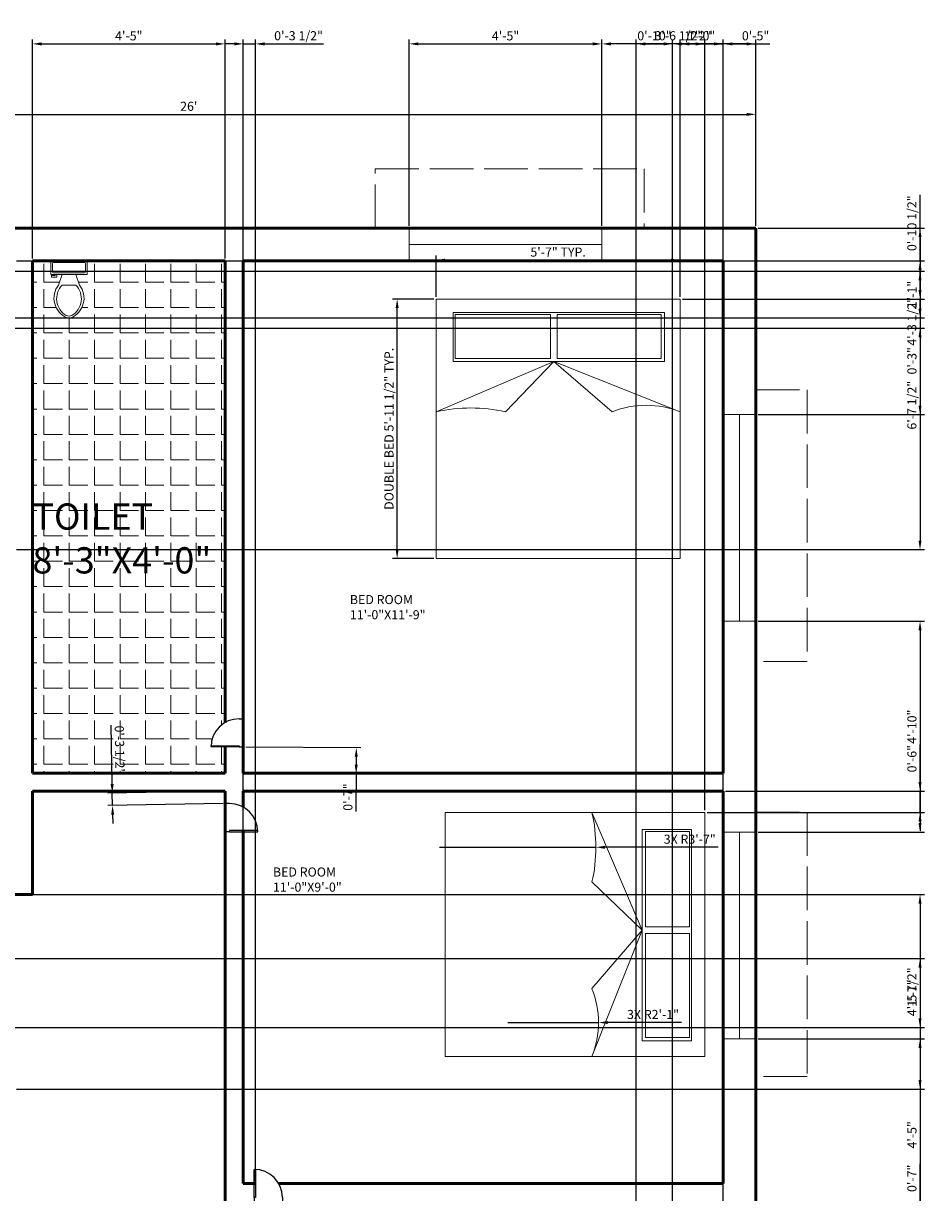
# Model space of a CAD drawing. Units: millimetres. Extents: x 3095 to 3505, y 1097 to 1734.
# Tile 5 of 5: x 3256 to 3505, y 1412 to 1734. Entities that reach past the tile are written whole.
import ezdxf

# ---------------------------------------------------------------- set-up
doc = ezdxf.new("R2010")
doc.units = ezdxf.units.MM
doc.linetypes.add('ACAD_ISO02W100', pattern=[15, 12, -3])
for name, color, linetype, lineweight, true_color in [('A-ANNO-DIMS', 32, 'Continuous', 18, 0xcd6928), ('A-AREA-IDEN', 152, 'Continuous', 18, 0x2776bb), ('A-FLOR-FIXT', 9, 'Continuous', 18, 0xafd9aa), ('A-FLOR-PATT', 241, 'Continuous', 13, 0xf7abae), ('A-FURN', 9, 'Continuous', 18, 0xafd9aa), ('A-GLAZ', 9, 'Continuous', 18, 0xd19cc7), ('A-ROOF-OVHD', 152, 'ACAD_ISO02W100', 13, 0x2776bb)]:
    doc.layers.add(name, color=color, linetype=linetype, lineweight=lineweight, true_color=true_color)
doc.layers.add('A-DOOR', color=4, linetype='Continuous', lineweight=25)
doc.layers.add('A-WALL', color=7, linetype='Continuous', lineweight=50)
doc.styles.get("Standard").update_dxf_attribs({"font": 'arial.ttf'})
doc.dimstyles.new('ISO-25', dxfattribs={"dimtxt": 2.5, "dimasz": 2.5, "dimexe": 1.25, "dimexo": 0.625, "dimtad": 1, "dimlunit": 3, "dimtxsty": 'Standard', "dimcen": 2.5, "dimadec": 0, "dimazin": 0, "dimtfac": 1, "dimtmove": 0, "dimatfit": 3, "dimfxl": 1, "dimarcsym": 0})

# ---------------------------------------------------------------- blocks, each defined once
blk = doc.blocks.new('*U4')
for p, q in [((9.5, -6), (9.5, -2)), ((-10, -8.5), (-8, -8.5)), ((-10, -9.5), (-10, -8.5)), ((-7, -9.5), (-10, -9.5)), ((-8, -8.5), (-8, -8)), ((-7, -8), (-7, -9.5)), ((-4, -8), (-6, -14)), ((4, -8), (6, -14)), ((4, -14), (-4, -14))]:
    blk.add_line(p, q)
blk.add_lwpolyline([(10.5, -8), (10.5, 0), (-10.5, 0), (-10.5, -8)], close=True)
for points in [[(-9.5, -2), (-9.5, -6)], [(8.5, -1), (-8.5, -1)], [(-8.5, -7), (8.5, -7)]]:
    blk.add_lwpolyline(points)
for centre, radius, start, end in [((-8.62, -1.88), 0.884, 81.8699, 188.1301), ((-8.62, -6.12), 0.884, 171.8699, 278.1301), ((8.62, -1.88), 0.884, 351.8699, 98.1301), ((8.62, -6.12), 0.884, 261.8699, 8.1301), ((3.52, -21.58), 12.17, 141.46911, 247.97143), ((4.2, -21.82), 11.33, 136.36773, 238.94682), ((-3.52, -21.58), 12.17, 292.02843, 38.53071), ((-4.2, -21.82), 11.33, 301.05301, 43.63209), ((0, -27.88), 4, 245.73182, 294.26817), ((0, -29), 4, 254.86053, 285.13947)]:
    blk.add_arc(centre, radius, start, end)
blk = doc.blocks.new('*U6')
for p, q in [((0, 0), (0, -6)), ((40, 0), (40, -6))]:
    blk.add_line(p, q)
blk.add_lwpolyline([(0, 0), (0, 40), (1.75, 40), (1.75, 0)], close=True)
blk.add_arc((0, 0), 40, 0, 90)
blk = doc.blocks.new('*U7')
for p, q in [((0, 0), (0, -6)), ((-40, 0), (-40, -6))]:
    blk.add_line(p, q)
blk.add_lwpolyline([(0, 0), (0, 40), (-1.75, 40), (-1.75, 0)], close=True)
blk.add_arc((0, 0), 40, 90, 180)
blk = doc.blocks.new('*D10')
at = {"layer": 'A-ANNO-DIMS', "color": 0, "lineweight": -2, "transparency": 16777216}
for p, q in [((3145.86, 1677.94), (3145.86, 1709.87)), ((3457.86, 1677.94), (3457.86, 1709.87)), ((3148.36, 1708.62), (3455.36, 1708.62))]:
    blk.add_line(p, q, dxfattribs=at)
at = {"layer": 'A-ANNO-DIMS', "color": 0, "lineweight": 5, "transparency": 16777216}
for points in [[(3148.36, 1709.03), (3148.36, 1708.2), (3145.86, 1708.62)], [(3455.36, 1709.03), (3455.36, 1708.2), (3457.86, 1708.62)]]:
    blk.add_solid(points, dxfattribs=at)
at = {"layer": 'Defpoints', "color": 0, "lineweight": 5, "transparency": 16777216}
for p in [(3457.86, 1708.62), (3145.86, 1677.32), (3457.86, 1677.32)]:
    blk.add_point(p, dxfattribs=at)
at = {"layer": 'A-ANNO-DIMS', "color": 0, "transparency": 16777216, "insert": (3301.86, 1710.52), "char_height": 2.5, "attachment_point": 5}
blk.add_mtext("26'", dxfattribs=at)
blk = doc.blocks.new('BED-DOUBLE')
for p, q in [((4.67, 67.71), (4.67, 54.2)), ((4.67, 67.71), (62.81, 67.71)), ((62.81, 54.2), (62.81, 67.71)), ((32.4, 54.2), (0, 40.37)), ((4.67, 54.2), (62.81, 54.2)), ((32.4, 54.2), (19.1, 40.37)), ((67.13, 40.37), (32.4, 54.2)), ((32.4, 54.2), (48.47, 40.37))]:
    blk.add_line(p, q)
for points in [[(0, 71.42), (67.13, 71.42), (67.13, 0), (0, 0)], [(5.23, 67.2), (31.46, 67.2), (31.46, 55.05), (5.23, 55.05)], [(33.33, 67.2), (61.88, 67.2), (61.88, 55.05), (33.33, 55.05)]]:
    blk.add_lwpolyline(points, close=True)
for centre, radius, start, end in [((57.8, 17.19), 24.99, 68.0833, 111.9167), ((9.55, -1.59), 43.03, 77.1763, 102.8237)]:
    blk.add_arc(centre, radius, start, end)
blk = doc.blocks.new('WIN-BEDROOM')
for p, q in [((0, 56.87), (9, 56.87)), ((0, 0), (0, 56.87)), ((0, 56.87), (4.5, 56.87)), ((4.5, 56.87), (4.5, 0)), ((9, 56.87), (9, 0)), ((9, 0), (0, 0))]:
    blk.add_line(p, q)
blk = doc.blocks.new('*D18')
at = {"layer": 'A-ANNO-DIMS', "color": 0, "lineweight": -2, "transparency": 16777216}
for p, q in [((3369.28, 1657.78), (3357.94, 1657.78)), ((3359.19, 1588.86), (3359.19, 1655.28)), ((3369.28, 1586.36), (3357.94, 1586.36))]:
    blk.add_line(p, q, dxfattribs=at)
at = {"layer": 'A-ANNO-DIMS', "color": 0, "lineweight": 5, "transparency": 16777216}
for points in [[(3358.77, 1655.28), (3359.61, 1655.28), (3359.19, 1657.78)], [(3358.77, 1588.86), (3359.61, 1588.86), (3359.19, 1586.36)]]:
    blk.add_solid(points, dxfattribs=at)
at = {"layer": 'Defpoints', "color": 0, "lineweight": 5, "transparency": 16777216}
for p in [(3359.19, 1657.78), (3369.9, 1657.78), (3369.9, 1586.36)]:
    blk.add_point(p, dxfattribs=at)
at = {"layer": 'A-ANNO-DIMS', "color": 0, "transparency": 16777216, "insert": (3357.27, 1622.07), "char_height": 2.5, "attachment_point": 5, "rotation": 90}
blk.add_mtext('DOUBLE BED 5\'-11 1/2" TYP.', dxfattribs=at)
blk = doc.blocks.new('*D19')
at = {"layer": 'A-ANNO-DIMS', "color": 0, "lineweight": -2, "transparency": 16777216}
for p, q in [((3369.9, 1658.41), (3369.9, 1669.75)), ((3372.4, 1668.5), (3434.53, 1668.5)), ((3437.03, 1658.41), (3437.03, 1669.75))]:
    blk.add_line(p, q, dxfattribs=at)
at = {"layer": 'A-ANNO-DIMS', "color": 0, "lineweight": 5, "transparency": 16777216}
for points in [[(3372.4, 1668.91), (3372.4, 1668.08), (3369.9, 1668.5)], [(3434.53, 1668.91), (3434.53, 1668.08), (3437.03, 1668.5)]]:
    blk.add_solid(points, dxfattribs=at)
at = {"layer": 'Defpoints', "color": 0, "lineweight": 5, "transparency": 16777216}
for p in [(3437.03, 1668.5), (3369.9, 1657.78), (3437.03, 1657.78)]:
    blk.add_point(p, dxfattribs=at)
at = {"layer": 'A-ANNO-DIMS', "color": 0, "transparency": 16777216, "insert": (3403.47, 1670.39), "char_height": 2.5, "attachment_point": 5}
blk.add_mtext('5\'-7" TYP.', dxfattribs=at)
blk = doc.blocks.new('*D32')
at = {"layer": 'A-ANNO-DIMS', "color": 0, "lineweight": -2, "transparency": 16777216}
for p, q in [((3415.51, 1677.94), (3415.51, 1729.27)), ((3457.86, 1677.94), (3457.86, 1729.27)), ((3455.36, 1728.02), (3418.01, 1728.02))]:
    blk.add_line(p, q, dxfattribs=at)
at = {"layer": 'A-ANNO-DIMS', "color": 0, "lineweight": 5, "transparency": 16777216}
for points in [[(3418.01, 1728.43), (3418.01, 1727.6), (3415.51, 1728.02)], [(3455.36, 1728.43), (3455.36, 1727.6), (3457.86, 1728.02)]]:
    blk.add_solid(points, dxfattribs=at)
at = {"layer": 'Defpoints', "color": 0, "lineweight": 5, "transparency": 16777216}
for p in [(3415.51, 1728.02), (3415.51, 1677.32), (3457.86, 1677.32)]:
    blk.add_point(p, dxfattribs=at)
at = {"layer": 'A-ANNO-DIMS', "color": 0, "transparency": 16777216, "insert": (3436.69, 1729.94), "char_height": 2.5, "attachment_point": 5}
blk.add_mtext('3\'-6 1/2"', dxfattribs=at)
blk = doc.blocks.new('*D33')
at = {"layer": 'A-ANNO-DIMS', "color": 0, "lineweight": -2, "transparency": 16777216}
for p, q in [((3362.52, 1677.94), (3362.52, 1729.27)), ((3415.51, 1677.94), (3415.51, 1729.27)), ((3365.02, 1728.02), (3413.01, 1728.02))]:
    blk.add_line(p, q, dxfattribs=at)
at = {"layer": 'A-ANNO-DIMS', "color": 0, "lineweight": 5, "transparency": 16777216}
for points in [[(3365.02, 1728.43), (3365.02, 1727.6), (3362.52, 1728.02)], [(3413.01, 1728.43), (3413.01, 1727.6), (3415.51, 1728.02)]]:
    blk.add_solid(points, dxfattribs=at)
at = {"layer": 'Defpoints', "color": 0, "lineweight": 5, "transparency": 16777216}
for p in [(3415.51, 1728.02), (3362.52, 1677.32), (3415.51, 1677.32)]:
    blk.add_point(p, dxfattribs=at)
at = {"layer": 'A-ANNO-DIMS', "color": 0, "transparency": 16777216, "insert": (3389.01, 1729.91), "char_height": 2.5, "attachment_point": 5}
blk.add_mtext('4\'-5"', dxfattribs=at)
blk = doc.blocks.new('*D38')
at = {"layer": 'A-ANNO-DIMS', "color": 0, "lineweight": -2, "transparency": 16777216}
for p, q in [((3458.49, 1677.32), (3504.29, 1677.32)), ((3503.04, 1674.82), (3503.04, 1628.48)), ((3458.49, 1625.98), (3504.29, 1625.98))]:
    blk.add_line(p, q, dxfattribs=at)
at = {"layer": 'A-ANNO-DIMS', "color": 0, "lineweight": 5, "transparency": 16777216}
for points in [[(3502.63, 1674.82), (3503.46, 1674.82), (3503.04, 1677.32)], [(3502.63, 1628.48), (3503.46, 1628.48), (3503.04, 1625.98)]]:
    blk.add_solid(points, dxfattribs=at)
at = {"layer": 'Defpoints', "color": 0, "lineweight": 5, "transparency": 16777216}
for p in [(3457.86, 1677.32), (3457.86, 1625.98), (3503.04, 1625.98)]:
    blk.add_point(p, dxfattribs=at)
at = {"layer": 'A-ANNO-DIMS', "color": 0, "transparency": 16777216, "insert": (3501.12, 1651.65), "char_height": 2.5, "attachment_point": 5, "rotation": 90}
blk.add_mtext('4\'-3 1/2"', dxfattribs=at)
blk = doc.blocks.new('*D39')
at = {"layer": 'A-ANNO-DIMS', "color": 0, "lineweight": -2, "transparency": 16777216}
for p, q in [((3458.49, 1569.11), (3504.29, 1569.11)), ((3503.04, 1566.61), (3503.04, 1513.53)), ((3458.49, 1511.03), (3504.29, 1511.03))]:
    blk.add_line(p, q, dxfattribs=at)
at = {"layer": 'A-ANNO-DIMS', "color": 0, "lineweight": 5, "transparency": 16777216}
for points in [[(3502.63, 1566.61), (3503.46, 1566.61), (3503.04, 1569.11)], [(3502.63, 1513.53), (3503.46, 1513.53), (3503.04, 1511.03)]]:
    blk.add_solid(points, dxfattribs=at)
at = {"layer": 'Defpoints', "color": 0, "lineweight": 5, "transparency": 16777216}
for p in [(3457.86, 1569.11), (3457.86, 1511.03), (3503.04, 1511.03)]:
    blk.add_point(p, dxfattribs=at)
at = {"layer": 'A-ANNO-DIMS', "color": 0, "transparency": 16777216, "insert": (3501.14, 1540.07), "char_height": 2.5, "attachment_point": 5, "rotation": 90}
blk.add_mtext('4\'-10"', dxfattribs=at)
blk = doc.blocks.new('*D40')
at = {"layer": 'A-ANNO-DIMS', "color": 0, "lineweight": -2, "transparency": 16777216}
for p, q in [((3458.49, 1454.16), (3504.29, 1454.16)), ((3503.04, 1451.66), (3503.04, 1403.79)), ((3458.49, 1401.29), (3504.29, 1401.29))]:
    blk.add_line(p, q, dxfattribs=at)
at = {"layer": 'A-ANNO-DIMS', "color": 0, "lineweight": 5, "transparency": 16777216}
for points in [[(3502.63, 1451.66), (3503.46, 1451.66), (3503.04, 1454.16)], [(3502.63, 1403.79), (3503.46, 1403.79), (3503.04, 1401.29)]]:
    blk.add_solid(points, dxfattribs=at)
at = {"layer": 'Defpoints', "color": 0, "lineweight": 5, "transparency": 16777216}
for p in [(3457.86, 1454.16), (3457.86, 1401.29), (3503.04, 1401.29)]:
    blk.add_point(p, dxfattribs=at)
at = {"layer": 'A-ANNO-DIMS', "color": 0, "transparency": 16777216, "insert": (3501.15, 1427.72), "char_height": 2.5, "attachment_point": 5, "rotation": 90}
blk.add_mtext('4\'-5"', dxfattribs=at)
blk = doc.blocks.new('*D45')
at = {"layer": 'A-ANNO-DIMS', "color": 0, "lineweight": -2, "transparency": 16777216}
for p, q in [((3258.86, 1668.94), (3258.86, 1729.27)), ((3311.86, 1668.94), (3311.86, 1729.27)), ((3261.36, 1728.02), (3309.36, 1728.02))]:
    blk.add_line(p, q, dxfattribs=at)
at = {"layer": 'A-ANNO-DIMS', "color": 0, "lineweight": 5, "transparency": 16777216}
for points in [[(3261.36, 1728.43), (3261.36, 1727.6), (3258.86, 1728.02)], [(3309.36, 1728.43), (3309.36, 1727.6), (3311.86, 1728.02)]]:
    blk.add_solid(points, dxfattribs=at)
at = {"layer": 'Defpoints', "color": 0, "lineweight": 5, "transparency": 16777216}
for p in [(3311.86, 1728.02), (3258.86, 1668.32), (3311.86, 1668.32)]:
    blk.add_point(p, dxfattribs=at)
at = {"layer": 'A-ANNO-DIMS', "color": 0, "transparency": 16777216, "insert": (3285.36, 1729.91), "char_height": 2.5, "attachment_point": 5}
blk.add_mtext('4\'-5"', dxfattribs=at)
blk = doc.blocks.new('*D48')
at = {"layer": 'A-ANNO-DIMS', "color": 0, "lineweight": -2, "transparency": 16777216}
for p, q in [((3254.49, 1668.32), (3504.29, 1668.32)), ((3503.04, 1665.82), (3503.04, 1591.3)), ((3254.49, 1588.8), (3504.29, 1588.8))]:
    blk.add_line(p, q, dxfattribs=at)
at = {"layer": 'A-ANNO-DIMS', "color": 0, "lineweight": 5, "transparency": 16777216}
for points in [[(3502.63, 1665.82), (3503.46, 1665.82), (3503.04, 1668.32)], [(3502.63, 1591.3), (3503.46, 1591.3), (3503.04, 1588.8)]]:
    blk.add_solid(points, dxfattribs=at)
at = {"layer": 'Defpoints', "color": 0, "lineweight": 5, "transparency": 16777216}
for p in [(3253.86, 1668.32), (3253.86, 1588.8), (3503.04, 1588.8)]:
    blk.add_point(p, dxfattribs=at)
at = {"layer": 'A-ANNO-DIMS', "color": 0, "transparency": 16777216, "insert": (3501.13, 1628.56), "char_height": 2.5, "attachment_point": 5, "rotation": 90}
blk.add_mtext('6\'-7 1/2"', dxfattribs=at)
blk = doc.blocks.new('*D53')
at = {"layer": 'A-ANNO-DIMS', "color": 0, "lineweight": -2, "transparency": 16777216}
for p, q in [((3232.89, 1476.25), (3504.29, 1476.25)), ((3503.04, 1473.75), (3503.04, 1459.75)), ((3232.89, 1457.25), (3504.29, 1457.25))]:
    blk.add_line(p, q, dxfattribs=at)
at = {"layer": 'A-ANNO-DIMS', "color": 0, "lineweight": 5, "transparency": 16777216}
for points in [[(3502.63, 1473.75), (3503.46, 1473.75), (3503.04, 1476.25)], [(3502.63, 1459.75), (3503.46, 1459.75), (3503.04, 1457.25)]]:
    blk.add_solid(points, dxfattribs=at)
at = {"layer": 'Defpoints', "color": 0, "lineweight": 5, "transparency": 16777216}
for p in [(3232.26, 1476.25), (3232.26, 1457.25), (3503.04, 1457.25)]:
    blk.add_point(p, dxfattribs=at)
at = {"layer": 'A-ANNO-DIMS', "color": 0, "transparency": 16777216, "insert": (3501.16, 1466.75), "char_height": 2.5, "attachment_point": 5, "rotation": 90}
blk.add_mtext('1\'-7"', dxfattribs=at)
blk = doc.blocks.new('*D54')
at = {"layer": 'A-ANNO-DIMS', "color": 0, "lineweight": -2, "transparency": 16777216}
for p, q in [((3254.49, 1493.86), (3504.29, 1493.86)), ((3503.04, 1491.36), (3503.04, 1442.82)), ((3254.49, 1440.32), (3504.29, 1440.32))]:
    blk.add_line(p, q, dxfattribs=at)
at = {"layer": 'A-ANNO-DIMS', "color": 0, "lineweight": 5, "transparency": 16777216}
for points in [[(3502.63, 1491.36), (3503.46, 1491.36), (3503.04, 1493.86)], [(3502.63, 1442.82), (3503.46, 1442.82), (3503.04, 1440.32)]]:
    blk.add_solid(points, dxfattribs=at)
at = {"layer": 'Defpoints', "color": 0, "lineweight": 5, "transparency": 16777216}
for p in [(3253.86, 1493.86), (3253.86, 1440.32), (3503.04, 1440.32)]:
    blk.add_point(p, dxfattribs=at)
at = {"layer": 'A-ANNO-DIMS', "color": 0, "transparency": 16777216, "insert": (3501.13, 1467.09), "char_height": 2.5, "attachment_point": 5, "rotation": 90}
blk.add_mtext('4\'-5 1/2"', dxfattribs=at)
blk = doc.blocks.new('*D56')
at = {"layer": 'A-ANNO-DIMS', "color": 0, "lineweight": -2, "transparency": 16777216}
for p, q in [((3211.99, 1665.48), (3504.29, 1665.48)), ((3503.04, 1662.98), (3503.04, 1655.1)), ((3211.99, 1652.6), (3504.29, 1652.6))]:
    blk.add_line(p, q, dxfattribs=at)
at = {"layer": 'A-ANNO-DIMS', "color": 0, "lineweight": 5, "transparency": 16777216}
for points in [[(3502.63, 1662.98), (3503.46, 1662.98), (3503.04, 1665.48)], [(3502.63, 1655.1), (3503.46, 1655.1), (3503.04, 1652.6)]]:
    blk.add_solid(points, dxfattribs=at)
at = {"layer": 'Defpoints', "color": 0, "lineweight": 5, "transparency": 16777216}
for p in [(3211.36, 1665.48), (3211.36, 1652.6), (3503.04, 1652.6)]:
    blk.add_point(p, dxfattribs=at)
at = {"layer": 'A-ANNO-DIMS', "color": 0, "transparency": 16777216, "insert": (3501.16, 1659.04), "char_height": 2.5, "attachment_point": 5, "rotation": 90}
blk.add_mtext('1\'-1"', dxfattribs=at)
blk = doc.blocks.new('*D59')
at = {"layer": 'A-ANNO-DIMS', "color": 0, "lineweight": -2, "transparency": 16777216}
for p, q in [((3424.96, 1366.94), (3424.96, 1729.27)), ((3434.99, 1366.94), (3434.99, 1729.27)), ((3427.46, 1728.02), (3432.49, 1728.02))]:
    blk.add_line(p, q, dxfattribs=at)
at = {"layer": 'A-ANNO-DIMS', "color": 0, "lineweight": 5, "transparency": 16777216}
for points in [[(3427.46, 1728.43), (3427.46, 1727.6), (3424.96, 1728.02)], [(3432.49, 1728.43), (3432.49, 1727.6), (3434.99, 1728.02)]]:
    blk.add_solid(points, dxfattribs=at)
at = {"layer": 'Defpoints', "color": 0, "lineweight": 5, "transparency": 16777216}
for p in [(3434.99, 1728.02), (3424.96, 1366.32), (3434.99, 1366.32)]:
    blk.add_point(p, dxfattribs=at)
at = {"layer": 'A-ANNO-DIMS', "color": 0, "transparency": 16777216, "insert": (3429.98, 1729.92), "char_height": 2.5, "attachment_point": 5}
blk.add_mtext('0\'-10"', dxfattribs=at)
blk = doc.blocks.new('*D61')
at = {"layer": 'A-ANNO-DIMS', "color": 0, "lineweight": -2, "transparency": 16777216}
for p, q in [((3434.99, 1366.94), (3434.99, 1729.27)), ((3448.86, 1366.94), (3448.86, 1729.27)), ((3437.49, 1728.02), (3446.36, 1728.02))]:
    blk.add_line(p, q, dxfattribs=at)
at = {"layer": 'A-ANNO-DIMS', "color": 0, "lineweight": 5, "transparency": 16777216}
for points in [[(3437.49, 1728.43), (3437.49, 1727.6), (3434.99, 1728.02)], [(3446.36, 1728.43), (3446.36, 1727.6), (3448.86, 1728.02)]]:
    blk.add_solid(points, dxfattribs=at)
at = {"layer": 'Defpoints', "color": 0, "lineweight": 5, "transparency": 16777216}
for p in [(3448.86, 1728.02), (3434.99, 1366.32), (3448.86, 1366.32)]:
    blk.add_point(p, dxfattribs=at)
at = {"layer": 'A-ANNO-DIMS', "color": 0, "transparency": 16777216, "insert": (3441.93, 1729.9), "char_height": 2.5, "attachment_point": 5}
blk.add_mtext('1\'-2"', dxfattribs=at)
blk = doc.blocks.new('*D63')
at = {"layer": 'A-ANNO-DIMS', "color": 0, "lineweight": -2, "transparency": 16777216}
for p, q in [((3503.04, 1409.32), (3503.04, 1419.71)), ((3356.49, 1409.32), (3504.29, 1409.32)), ((3503.04, 1404.64), (3503.04, 1406.82)), ((3356.49, 1402.14), (3504.29, 1402.14))]:
    blk.add_line(p, q, dxfattribs=at)
at = {"layer": 'A-ANNO-DIMS', "color": 0, "lineweight": 5, "transparency": 16777216}
for points in [[(3502.63, 1406.82), (3503.46, 1406.82), (3503.04, 1409.32)], [(3502.63, 1404.64), (3503.46, 1404.64), (3503.04, 1402.14)]]:
    blk.add_solid(points, dxfattribs=at)
at = {"layer": 'Defpoints', "color": 0, "lineweight": 5, "transparency": 16777216}
for p in [(3355.86, 1409.32), (3503.04, 1409.32), (3355.86, 1402.14)]:
    blk.add_point(p, dxfattribs=at)
at = {"layer": 'A-ANNO-DIMS', "color": 0, "transparency": 16777216, "insert": (3501.14, 1415.76), "char_height": 2.5, "attachment_point": 5, "rotation": 90}
blk.add_mtext('0\'-7"', dxfattribs=at)
blk = doc.blocks.new('*D73')
at = {"layer": 'A-ANNO-DIMS', "color": 0, "lineweight": -2, "transparency": 16777216}
for p, q in [((3503.04, 1655.1), (3503.04, 1657.6)), ((3211.99, 1652.6), (3504.29, 1652.6)), ((3503.04, 1652.6), (3503.04, 1649.73)), ((3222.62, 1649.73), (3504.29, 1649.73)), ((3503.04, 1647.23), (3503.04, 1636.83))]:
    blk.add_line(p, q, dxfattribs=at)
at = {"layer": 'A-ANNO-DIMS', "color": 0, "lineweight": 5, "transparency": 16777216}
for points in [[(3502.63, 1655.1), (3503.46, 1655.1), (3503.04, 1652.6)], [(3502.63, 1647.23), (3503.46, 1647.23), (3503.04, 1649.73)]]:
    blk.add_solid(points, dxfattribs=at)
at = {"layer": 'Defpoints', "color": 0, "lineweight": 5, "transparency": 16777216}
for p in [(3211.36, 1652.6), (3222, 1649.73), (3503.04, 1649.73)]:
    blk.add_point(p, dxfattribs=at)
at = {"layer": 'A-ANNO-DIMS', "color": 0, "transparency": 16777216, "insert": (3501.14, 1640.78), "char_height": 2.5, "attachment_point": 5, "rotation": 90}
blk.add_mtext('0\'-3"', dxfattribs=at)
blk = doc.blocks.new('*D78')
at = {"layer": 'A-ANNO-DIMS', "color": 0, "lineweight": -2, "transparency": 16777216}
for p, q in [((3437.03, 1658.41), (3437.03, 1729.27)), ((3448.86, 1668.94), (3448.86, 1729.27)), ((3439.53, 1728.02), (3446.36, 1728.02))]:
    blk.add_line(p, q, dxfattribs=at)
at = {"layer": 'A-ANNO-DIMS', "color": 0, "lineweight": 5, "transparency": 16777216}
for points in [[(3439.53, 1728.43), (3439.53, 1727.6), (3437.03, 1728.02)], [(3446.36, 1728.43), (3446.36, 1727.6), (3448.86, 1728.02)]]:
    blk.add_solid(points, dxfattribs=at)
at = {"layer": 'Defpoints', "color": 0, "lineweight": 5, "transparency": 16777216}
for p in [(3448.86, 1728.02), (3448.86, 1668.32), (3437.03, 1657.78)]:
    blk.add_point(p, dxfattribs=at)
at = {"layer": 'A-ANNO-DIMS', "color": 0, "transparency": 16777216, "insert": (3442.95, 1729.92), "char_height": 2.5, "attachment_point": 5}
blk.add_mtext('1\'-0"', dxfattribs=at)
blk = doc.blocks.new('*D79')
at = {"layer": 'A-ANNO-DIMS', "color": 0, "lineweight": -2, "transparency": 16777216}
for p, q in [((3503.04, 1668.32), (3503.04, 1686.48)), ((3449.49, 1668.32), (3504.29, 1668.32)), ((3503.04, 1660.28), (3503.04, 1665.82)), ((3437.65, 1657.78), (3504.29, 1657.78))]:
    blk.add_line(p, q, dxfattribs=at)
at = {"layer": 'A-ANNO-DIMS', "color": 0, "lineweight": 5, "transparency": 16777216}
for points in [[(3502.63, 1665.82), (3503.46, 1665.82), (3503.04, 1668.32)], [(3502.63, 1660.28), (3503.46, 1660.28), (3503.04, 1657.78)]]:
    blk.add_solid(points, dxfattribs=at)
at = {"layer": 'Defpoints', "color": 0, "lineweight": 5, "transparency": 16777216}
for p in [(3448.86, 1668.32), (3503.04, 1668.32), (3437.03, 1657.78)]:
    blk.add_point(p, dxfattribs=at)
at = {"layer": 'A-ANNO-DIMS', "color": 0, "transparency": 16777216, "insert": (3501.13, 1678.65), "char_height": 2.5, "attachment_point": 5, "rotation": 90}
blk.add_mtext('0\'-10 1/2"', dxfattribs=at)
blk = doc.blocks.new('*D81')
at = {"layer": 'A-ANNO-DIMS', "color": 0, "lineweight": -2, "transparency": 16777216}
for p, q in [((3317.53, 1534.49), (3349.2, 1534.3)), ((3347.94, 1531.81), (3347.93, 1529.63)), ((3317.49, 1527.31), (3349.16, 1527.12)), ((3347.91, 1527.13), (3347.85, 1516.74))]:
    blk.add_line(p, q, dxfattribs=at)
at = {"layer": 'A-ANNO-DIMS', "color": 0, "lineweight": 5, "transparency": 16777216}
for points in [[(3347.52, 1531.81), (3348.36, 1531.8), (3347.95, 1534.31)], [(3347.51, 1529.63), (3348.34, 1529.63), (3347.91, 1527.13)]]:
    blk.add_solid(points, dxfattribs=at)
at = {"layer": 'Defpoints', "color": 0, "lineweight": 5, "transparency": 16777216}
for p in [(3316.91, 1534.49), (3316.86, 1527.32), (3347.91, 1527.13)]:
    blk.add_point(p, dxfattribs=at)
at = {"layer": 'A-ANNO-DIMS', "color": 0, "transparency": 16777216, "insert": (3345.97, 1520.69), "char_height": 2.5, "attachment_point": 5, "rotation": 89.6578}
blk.add_mtext('0\'-7"', dxfattribs=at)
blk = doc.blocks.new('*D82')
at = {"layer": 'A-ANNO-DIMS', "color": 0, "lineweight": -2, "transparency": 16777216}
for p, q in [((3280.77, 1524.28), (3280.49, 1540.49)), ((3311.24, 1522.31), (3279.57, 1521.75)), ((3280.88, 1518.38), (3280.82, 1521.78)), ((3311.3, 1518.91), (3279.63, 1518.36)), ((3280.92, 1515.88), (3280.96, 1513.38))]:
    blk.add_line(p, q, dxfattribs=at)
at = {"layer": 'A-ANNO-DIMS', "color": 0, "lineweight": 5, "transparency": 16777216}
for points in [[(3281.19, 1524.28), (3280.36, 1524.27), (3280.82, 1521.78)], [(3281.34, 1515.89), (3280.5, 1515.87), (3280.88, 1518.38)]]:
    blk.add_solid(points, dxfattribs=at)
at = {"layer": 'Defpoints', "color": 0, "lineweight": 5, "transparency": 16777216}
for p in [(3280.82, 1521.78), (3311.86, 1522.32), (3311.92, 1518.92)]:
    blk.add_point(p, dxfattribs=at)
at = {"layer": 'A-ANNO-DIMS', "color": 0, "transparency": 16777216, "insert": (3282.53, 1533.67), "char_height": 2.5, "attachment_point": 5, "rotation": 270.9972}
blk.add_mtext('0\'-3 1/2"', dxfattribs=at)
blk = doc.blocks.new('*D83')
at = {"layer": 'A-ANNO-DIMS', "color": 0, "lineweight": -2, "transparency": 16777216}
for p, q in [((3316.86, 1414.94), (3316.86, 1729.27)), ((3320.2, 1414.94), (3320.2, 1729.27)), ((3314.36, 1728.02), (3311.86, 1728.02)), ((3316.86, 1728.02), (3320.2, 1728.02)), ((3322.7, 1728.02), (3338.93, 1728.02))]:
    blk.add_line(p, q, dxfattribs=at)
at = {"layer": 'A-ANNO-DIMS', "color": 0, "lineweight": 5, "transparency": 16777216}
for points in [[(3314.36, 1728.43), (3314.36, 1727.6), (3316.86, 1728.02)], [(3322.7, 1728.43), (3322.7, 1727.6), (3320.2, 1728.02)]]:
    blk.add_solid(points, dxfattribs=at)
at = {"layer": 'Defpoints', "color": 0, "lineweight": 5, "transparency": 16777216}
for p in [(3320.2, 1728.02), (3316.86, 1414.32), (3320.2, 1414.32)]:
    blk.add_point(p, dxfattribs=at)
at = {"layer": 'A-ANNO-DIMS', "color": 0, "transparency": 16777216, "insert": (3332.06, 1729.94), "char_height": 2.5, "attachment_point": 5}
blk.add_mtext('0\'-3 1/2"', dxfattribs=at)
blk = doc.blocks.new('*D84')
at = {"layer": 'A-ANNO-DIMS', "color": 0, "lineweight": -2, "transparency": 16777216}
for p, q in [((3443.85, 1517.05), (3443.85, 1729.27)), ((3448.86, 1522.94), (3448.86, 1729.27)), ((3441.35, 1728.02), (3438.85, 1728.02)), ((3443.85, 1728.02), (3448.86, 1728.02)), ((3451.36, 1728.02), (3461.76, 1728.02))]:
    blk.add_line(p, q, dxfattribs=at)
at = {"layer": 'A-ANNO-DIMS', "color": 0, "lineweight": 5, "transparency": 16777216}
for points in [[(3441.35, 1728.43), (3441.35, 1727.6), (3443.85, 1728.02)], [(3451.36, 1728.43), (3451.36, 1727.6), (3448.86, 1728.02)]]:
    blk.add_solid(points, dxfattribs=at)
at = {"layer": 'Defpoints', "color": 0, "lineweight": 5, "transparency": 16777216}
for p in [(3448.86, 1728.02), (3448.86, 1522.32), (3443.85, 1516.43)]:
    blk.add_point(p, dxfattribs=at)
at = {"layer": 'A-ANNO-DIMS', "color": 0, "transparency": 16777216, "insert": (3457.81, 1729.92), "char_height": 2.5, "attachment_point": 5}
blk.add_mtext('0\'-5"', dxfattribs=at)
blk = doc.blocks.new('*D85')
at = {"layer": 'A-ANNO-DIMS', "color": 0, "lineweight": -2, "transparency": 16777216}
for p, q in [((3503.04, 1524.82), (3503.04, 1535.21)), ((3449.49, 1522.32), (3504.29, 1522.32)), ((3503.04, 1516.43), (3503.04, 1522.32)), ((3444.47, 1516.43), (3504.29, 1516.43)), ((3503.04, 1513.93), (3503.04, 1511.43))]:
    blk.add_line(p, q, dxfattribs=at)
at = {"layer": 'A-ANNO-DIMS', "color": 0, "lineweight": 5, "transparency": 16777216}
for points in [[(3502.63, 1524.82), (3503.46, 1524.82), (3503.04, 1522.32)], [(3502.63, 1513.93), (3503.46, 1513.93), (3503.04, 1516.43)]]:
    blk.add_solid(points, dxfattribs=at)
at = {"layer": 'Defpoints', "color": 0, "lineweight": 5, "transparency": 16777216}
for p in [(3448.86, 1522.32), (3503.04, 1522.32), (3443.85, 1516.43)]:
    blk.add_point(p, dxfattribs=at)
at = {"layer": 'A-ANNO-DIMS', "color": 0, "transparency": 16777216, "insert": (3501.14, 1531.26), "char_height": 2.5, "attachment_point": 5, "rotation": 90}
blk.add_mtext('0\'-6"', dxfattribs=at)
blk = doc.blocks.new('*D89')
at = {"layer": 'A-ANNO-DIMS', "color": 0, "lineweight": -2, "transparency": 16777216}
for p, q in [((3370.83, 1506.88), (3413.87, 1506.88)), ((3447.52, 1506.88), (3416.37, 1506.88))]:
    blk.add_line(p, q, dxfattribs=at)
at = {"layer": 'A-ANNO-DIMS', "color": 0, "lineweight": 5, "transparency": 16777216}
blk.add_solid([(3416.37, 1507.29), (3416.37, 1506.46), (3413.87, 1506.88)], dxfattribs=at)
at = {"layer": 'Defpoints', "color": 0, "lineweight": 5, "transparency": 16777216}
for p in [(3370.83, 1506.88), (3413.87, 1506.88)]:
    blk.add_point(p, dxfattribs=at)
at = {"layer": 'A-ANNO-DIMS', "color": 0, "transparency": 16777216, "insert": (3439.69, 1508.78), "char_height": 2.5, "attachment_point": 5, "rotation": 0.0007}
blk.add_mtext('3X R3\'-7"', dxfattribs=at)
blk = doc.blocks.new('*D90')
at = {"layer": 'A-ANNO-DIMS', "color": 0, "lineweight": -2, "transparency": 16777216}
for p, q in [((3389.61, 1458.63), (3414.6, 1458.63)), ((3437.42, 1458.63), (3417.1, 1458.63))]:
    blk.add_line(p, q, dxfattribs=at)
at = {"layer": 'A-ANNO-DIMS', "color": 0, "lineweight": 5, "transparency": 16777216}
blk.add_solid([(3417.1, 1459.04), (3417.1, 1458.21), (3414.6, 1458.63)], dxfattribs=at)
at = {"layer": 'Defpoints', "color": 0, "lineweight": 5, "transparency": 16777216}
for p in [(3389.61, 1458.63), (3414.6, 1458.63)]:
    blk.add_point(p, dxfattribs=at)
at = {"layer": 'A-ANNO-DIMS', "color": 0, "transparency": 16777216, "insert": (3429.59, 1460.53), "char_height": 2.5, "attachment_point": 5, "rotation": 359.9992}
blk.add_mtext('3X R2\'-1"', dxfattribs=at)

msp = doc.modelspace()

# ---------------------------------------------------------------- hatches: boundary and pattern name
at = {"layer": 'A-FLOR-PATT'}
h = msp.add_hatch(dxfattribs=at)
h.set_pattern_fill('ANGLE', color=256)
h.set_pattern_definition([(0, (0, 0), (0, 6.985), [5.08, -1.905]), (90, (0, 0), (-6.985, 4e-16), [5.08, -1.905])])
h.paths.add_polyline_path([(3311.862, 1668.316), (3273.923, 1668.316), (3273.923, 1664.496), (3270.819, 1664.496), (3271.774, 1661.631, -0.5301431), (3268.909, 1652.448, -0.530136), (3266.044, 1661.631), (3266.999, 1664.496), (3265.566, 1664.496), (3265.566, 1663.78), (3264.134, 1663.78), (3264.134, 1664.496), (3263.895, 1664.496), (3263.895, 1668.316), (3258.862, 1668.316), (3258.862, 1527.316), (3311.862, 1527.316), (3311.862, 1534.492), (3307.983, 1534.492), (3307.983, 1534.831), (3307.991, 1534.831, -0.2562565), (3311.862, 1541.211)])
h.paths.add_polyline_path([(3448.862, 1409.316), (3355.862, 1409.316), (3355.862, 1402.478), (3359.742, 1402.478), (3359.742, 1402.139), (3359.734, 1402.139, -0.2562565), (3355.862, 1395.759), (3355.862, 1366.316), (3424.964, 1366.316), (3424.964, 1370.136), (3428.068, 1370.136), (3427.113, 1373.001, -0.4652664), (3428.865, 1381.717, -0.3212229), (3431.09, 1381.717, -0.4652592), (3432.843, 1373.001), (3431.888, 1370.136), (3433.32, 1370.136), (3433.32, 1370.853), (3434.753, 1370.853), (3434.992, 1370.136), (3434.992, 1366.316), (3448.862, 1366.316)])
h.paths.add_polyline_path([(3428.308, 1345.964, -0.4652592), (3426.555, 1354.679), (3427.51, 1357.544), (3426.078, 1357.544), (3426.078, 1356.828), (3424.645, 1356.828), (3424.407, 1357.544), (3424.407, 1361.316), (3355.862, 1361.316), (3355.862, 1322.305, -0.0398063), (3357.095, 1322.349), (3357.095, 1322.357), (3356.756, 1322.357, -0.2743513), (3363.565, 1318.316), (3448.862, 1318.316), (3448.862, 1361.316), (3434.434, 1361.316), (3434.434, 1357.544), (3431.331, 1357.544), (3432.286, 1354.679, -0.4652664), (3430.533, 1345.964, -0.3212229)])

# ---------------------------------------------------------------- linework, layer by layer
at = {"layer": 'A-GLAZ'}
for p, q in [((3362.516, 1677.316), (3362.516, 1668.316)), ((3415.513, 1677.316), (3362.516, 1677.316)), ((3362.516, 1677.316), (3362.516, 1672.816)), ((3415.513, 1668.316), (3415.513, 1677.316)), ((3362.516, 1672.816), (3415.513, 1672.816)), ((3362.516, 1668.316), (3415.513, 1668.316))]:
    msp.add_line(p, q, dxfattribs=at)
at = {"layer": 'A-ROOF-OVHD'}
for p, q in [((3353.155, 1677.316), (3353.155, 1693.598)), ((3353.155, 1693.598), (3427.161, 1693.598)), ((3427.161, 1693.598), (3427.161, 1677.316)), ((3457.862, 1632.772), (3471.993, 1632.772)), ((3471.993, 1632.772), (3471.993, 1557.991)), ((3471.993, 1557.991), (3457.862, 1557.991)), ((3457.862, 1516.56), (3471.993, 1516.56)), ((3471.993, 1516.56), (3471.993, 1443.797)), ((3471.993, 1443.797), (3457.862, 1443.797))]:
    msp.add_line(p, q, dxfattribs=at)
at = {"layer": 'A-WALL'}
for p, q in [((3145.862, 1677.316), (3457.862, 1677.316)), ((3457.862, 1677.316), (3457.862, 1173.316)), ((3258.862, 1668.316), (3311.862, 1668.316)), ((3258.862, 1527.316), (3258.862, 1668.316)), ((3311.862, 1668.316), (3311.862, 1541.211)), ((3311.862, 1541.211), (3311.862, 1668.316)), ((3316.862, 1668.316), (3316.862, 1527.316)), ((3316.862, 1668.316), (3448.862, 1668.316)), ((3448.862, 1668.316), (3448.862, 1527.316)), ((3311.862, 1527.316), (3311.862, 1534.831)), ((3311.862, 1534.831), (3311.862, 1527.316)), ((3258.862, 1527.316), (3311.862, 1527.316)), ((3316.862, 1527.316), (3448.862, 1527.316)), ((3258.862, 1522.316), (3311.862, 1522.316)), ((3258.862, 1493.863), (3258.862, 1522.316)), ((3311.862, 1522.316), (3311.862, 1409.316)), ((3316.862, 1522.316), (3316.862, 1517.937)), ((3316.862, 1522.316), (3448.862, 1522.316)), ((3448.862, 1522.316), (3448.862, 1414.316)), ((3316.862, 1511.5), (3316.862, 1414.316)), ((3253.862, 1493.863), (3258.862, 1493.863)), ((3316.862, 1414.316), (3320.204, 1414.316)), ((3326.599, 1414.316), (3448.862, 1414.316))]:
    msp.add_line(p, q, dxfattribs=at)

# ---------------------------------------------------------------- block references
at = {"layer": 'A-DOOR', "xscale": 0.1939559161486229, "yscale": 0.1939559161486229, "zscale": 0.1939559161486229}
for name, p, rotation in [('*U6', (3315.742, 1534.492), 89.99999999999999), ('*U7', (3313.085, 1511.161), 270)]:
    msp.add_blockref(name, p, dxfattribs=dict(at, rotation=rotation))
msp.add_blockref('*U6', (3319.865, 1410.463), dxfattribs=at)
at = {"layer": 'A-FLOR-FIXT', "xscale": 0.4775205747460847, "yscale": 0.4775205747460847, "zscale": 0.4775205747460847}
msp.add_blockref('*U4', (3268.909, 1668.316), dxfattribs=at)
at = {"layer": 'A-FURN'}
msp.add_blockref('BED-DOUBLE', (3369.904, 1586.359), dxfattribs=at)
at = {"layer": 'A-FURN', "rotation": 270.0000000000001}
msp.add_blockref('BED-DOUBLE', (3372.422, 1516.427), dxfattribs=at)
at = {"layer": 'A-GLAZ'}
for p in [(3448.862, 1569.114), (3448.862, 1454.161)]:
    msp.add_blockref('WIN-BEDROOM', p, dxfattribs=at)

# ---------------------------------------------------------------- texts
at = {"layer": 'A-AREA-IDEN', "attachment_point": 1}
for s, width, gutter_width, insert, char_height in [('TOILET\\P8\'-3"X4\'-0"', 62.40222, 36.136, (3258.862, 1601.521), 7.22712), ('BED ROOM\\P11\'-0"X11\'-9"', 55.13748, 12.5, (3346.192, 1576.309), 2.5), ('BED ROOM\\P11\'-0"X9\'-0"', 47.39746, 12.5, (3325.024, 1501.316), 2.5)]:
    msp.add_mtext_dynamic_manual_height_columns(s, width=width, gutter_width=gutter_width, heights=[0], dxfattribs=dict(at, insert=insert, char_height=char_height))

# ---------------------------------------------------------------- dimensions: what is measured, and where the dimension line sits
at = {"layer": 'A-ANNO-DIMS'}
for base, p1, p2, override, picture, middle in [((3311.862, 1728.017), (3258.862, 1668.316), (3311.862, 1668.316), {"dimdec": 1, "dimlfac": 1, "dimrnd": 0, "dimzin": 1, "dimdsep": 46, "dimlunit": 4, "dimfrac": 2}, '*D45', (3285.362, 1729.914)), ((3320.204, 1728.017), (3316.862, 1414.316), (3320.204, 1414.316), {"dimdec": 1, "dimlfac": 1, "dimrnd": 0, "dimzin": 1, "dimdsep": 46, "dimlunit": 4, "dimfrac": 2}, '*D83', (3332.065, 1729.936)), ((3415.513, 1728.017), (3362.516, 1677.316), (3415.513, 1677.316), {"dimdec": 1, "dimlfac": 1, "dimrnd": 0, "dimzin": 1, "dimdsep": 46, "dimlunit": 4, "dimfrac": 2}, '*D33', (3389.015, 1729.914)), ((3415.513, 1728.017), (3457.862, 1677.316), (3415.513, 1677.316), {"dimdec": 1, "dimlfac": 1, "dimrnd": 0, "dimzin": 1, "dimdsep": 46, "dimlunit": 4, "dimfrac": 2}, '*D32', (3436.688, 1729.936)), ((3434.992, 1728.017), (3424.964, 1366.316), (3434.992, 1366.316), {"dimdec": 1, "dimlfac": 1, "dimrnd": 0, "dimzin": 1, "dimdsep": 46, "dimlunit": 4, "dimfrac": 2}, '*D59', (3429.978, 1729.919)), ((3448.862, 1728.017), (3434.992, 1366.316), (3448.862, 1366.316), {"dimdec": 1, "dimlfac": 1, "dimrnd": 0, "dimzin": 1, "dimdsep": 46, "dimlunit": 4, "dimfrac": 2}, '*D61', (3441.927, 1729.897)), ((3448.862, 1728.017), (3437.03, 1657.783), (3448.862, 1668.316), {"dimdec": 1, "dimlfac": 1, "dimrnd": 0, "dimzin": 1, "dimdsep": 46, "dimlunit": 4, "dimfrac": 2}, '*D78', (3442.946, 1729.919)), ((3448.862, 1728.017), (3443.846, 1516.427), (3448.862, 1522.316), {"dimdec": 1, "dimlfac": 1, "dimrnd": 0, "dimzin": 1, "dimdsep": 46, "dimlunit": 4, "dimfrac": 2}, '*D84', (3457.81, 1729.919)), ((3457.862, 1708.616), (3145.862, 1677.316), (3457.862, 1677.316), {"dimclrd": 0, "dimclre": 0, "dimclrt": 0}, '*D10', (3301.862, 1710.518))]:
    dim = msp.add_linear_dim(base=base, p1=p1, p2=p2, dimstyle='ISO-25', override=override, dxfattribs=at)
    dim.commit()
    dim.dimension.update_dxf_attribs({"geometry": picture, "text_midpoint": middle})
for base, p1, p2, angle, picture, middle in [((3503.043, 1668.316), (3437.03, 1657.783), (3448.862, 1668.316), 90, '*D79', (3501.125, 1678.648)), ((3503.043, 1625.98), (3457.862, 1677.316), (3457.862, 1625.98), 90, '*D38', (3501.124, 1651.648)), ((3503.043, 1588.796), (3253.862, 1668.316), (3253.862, 1588.796), 90, '*D48', (3501.125, 1628.556)), ((3503.043, 1652.599), (3211.364, 1665.476), (3211.364, 1652.599), 90, '*D56', (3501.163, 1659.038)), ((3503.043, 1649.727), (3211.364, 1652.599), (3221.995, 1649.727), 90, '*D73', (3501.141, 1640.78)), ((3503.043, 1511.027), (3457.862, 1569.114), (3457.862, 1511.027), 90, '*D39', (3501.141, 1540.07)), ((3280.817, 1521.776), (3311.922, 1518.919), (3311.862, 1522.316), 90.99723, '*D82', (3282.529, 1533.668)), ((3347.912, 1527.131), (3316.905, 1534.492), (3316.862, 1527.316), 269.65783, '*D81', (3345.972, 1520.694)), ((3503.043, 1522.316), (3443.846, 1516.427), (3448.862, 1522.316), 90, '*D85', (3501.141, 1531.264)), ((3503.043, 1440.316), (3253.862, 1493.863), (3253.862, 1440.316), 90, '*D54', (3501.125, 1467.09)), ((3503.043, 1457.251), (3232.262, 1476.252), (3232.262, 1457.251), 90, '*D53', (3501.163, 1466.752)), ((3503.043, 1401.286), (3457.862, 1454.161), (3457.862, 1401.286), 90, '*D40', (3501.147, 1427.723)), ((3503.043, 1409.316), (3355.862, 1402.139), (3355.862, 1409.316), 90, '*D63', (3501.141, 1415.764))]:
    dim = msp.add_linear_dim(base=base, p1=p1, p2=p2, angle=angle, dimstyle='ISO-25', override={"dimdec": 1, "dimlfac": 1, "dimrnd": 0, "dimzin": 1, "dimdsep": 46, "dimlunit": 4, "dimfrac": 2}, dxfattribs=at)
    dim.commit()
    dim.dimension.update_dxf_attribs({"geometry": picture, "text_midpoint": middle})
dim = msp.add_linear_dim(base=(3437.03, 1668.497), p1=(3369.904, 1657.783), p2=(3437.03, 1657.783), text='<> TYP.', dimstyle='ISO-25', override={"dimdec": 1, "dimlfac": 1, "dimrnd": 0, "dimzin": 1, "dimdsep": 46, "dimlunit": 4, "dimfrac": 2}, dxfattribs=at)
dim.commit()
dim.dimension.update_dxf_attribs({"geometry": '*D19', "text_midpoint": (3403.467, 1670.393)})
dim = msp.add_linear_dim(base=(3359.191, 1657.783), p1=(3369.904, 1586.359), p2=(3369.904, 1657.783), angle=90, text='DOUBLE BED <> TYP.', dimstyle='ISO-25', override={"dimdec": 1, "dimlfac": 1, "dimrnd": 0, "dimzin": 1, "dimdsep": 46, "dimlunit": 4, "dimfrac": 2}, dxfattribs=at)
dim.commit()
dim.dimension.update_dxf_attribs({"geometry": '*D18', "text_midpoint": (3357.272, 1622.071)})
for center, mpoint, picture, middle in [((3370.833, 1506.876), (3413.867, 1506.876), '*D89', (3439.687, 1506.876)), ((3389.612, 1458.628), (3414.6, 1458.628), '*D90', (3429.592, 1458.628))]:
    dim = msp.add_radius_dim(center=center, mpoint=mpoint, text='3X <>', dimstyle='ISO-25', override={"dimdec": 1, "dimlfac": 1, "dimrnd": 0, "dimzin": 1, "dimdsep": 46, "dimlunit": 4, "dimfrac": 2}, dxfattribs=at)
    dim.commit()
    dim.dimension.update_dxf_attribs({"geometry": picture, "text_midpoint": middle, "dimtype": 164})

doc.saveas('drawing.dxf')
